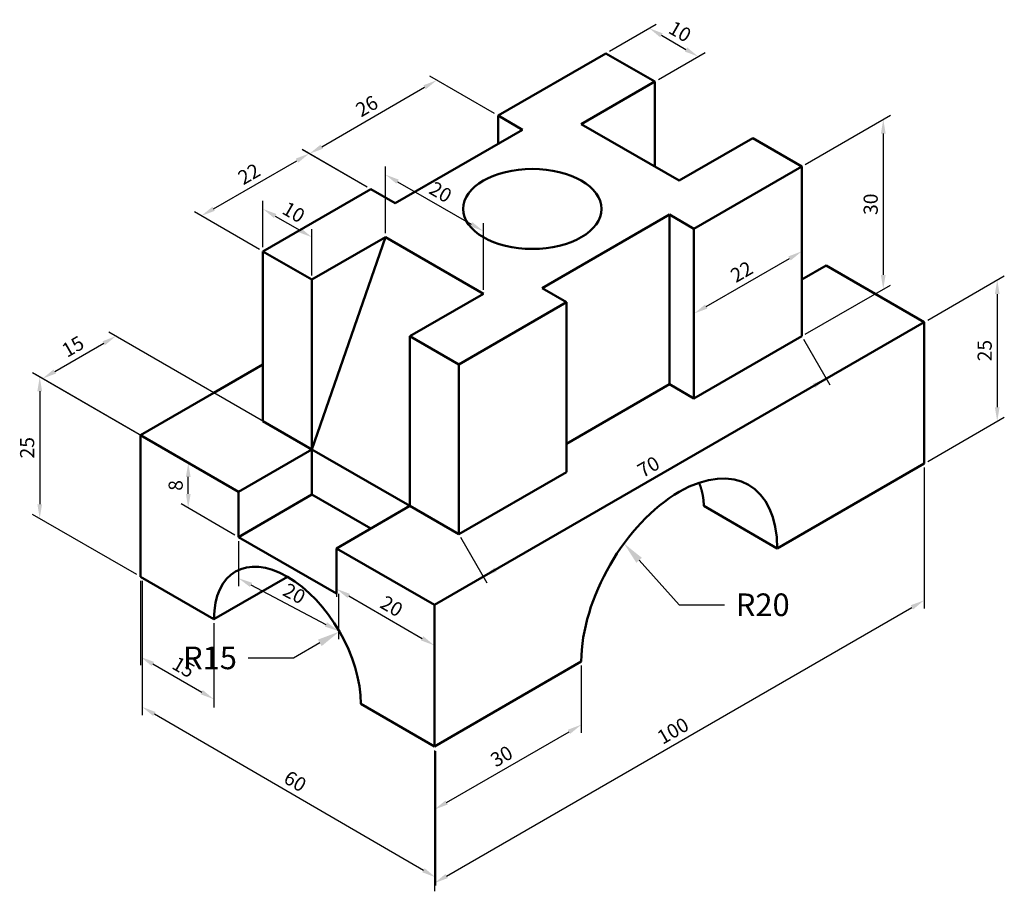
# Model space of a CAD drawing. Units: millimetres. Extents: x 69 to 243, y -4 to 150.
import ezdxf
from ezdxf import colors
from ezdxf.entities.mleader import LeaderData, LeaderLine
from ezdxf.math import Vec2, Vec3

# ---------------------------------------------------------------- set-up
doc = ezdxf.new("R2010")
doc.units = ezdxf.units.MM
for name, color, linetype, lineweight in [('M-DIMS', 3, 'Continuous', 25), ('M-OUTL', 7, 'Continuous', 50), ('M-TEXT', 3, 'Continuous', 25)]:
    doc.layers.add(name, color=color, linetype=linetype, lineweight=lineweight)
doc.styles.get("Standard").update_dxf_attribs({"font": 'arial.ttf'})
doc.dimstyles.new('ISO-25', dxfattribs={"dimtxt": 2.5, "dimasz": 2.5, "dimexe": 1.25, "dimexo": 0.625, "dimtad": 1, "dimtxsty": 'Standard', "dimcen": 2.5, "dimadec": 0, "dimazin": 0, "dimtfac": 1, "dimtmove": 0, "dimatfit": 3, "dimfxl": 1, "dimarcsym": 0})

# ---------------------------------------------------------------- blocks, each defined once
blk = doc.blocks.new('*D1')
at = {"layer": 'Defpoints', "color": 0, "transparency": 16777216}
for p in [(90.55, 76.18), (72.73, 61.47), (90.55, 51.18)]:
    blk.add_point(p, dxfattribs=at)
at = {"layer": 'M-DIMS', "color": 0, "lineweight": -2, "transparency": 16777216}
for p, q in [((89.92, 76.54), (71.48, 87.19)), ((72.73, 83.97), (72.73, 63.97)), ((89.92, 51.54), (71.48, 62.19))]:
    blk.add_line(p, q, dxfattribs=at)
at = {"layer": 'M-DIMS', "color": 0, "transparency": 16777216}
for points in [[(72.32, 83.97), (73.15, 83.97), (72.73, 86.47)], [(72.32, 63.97), (73.15, 63.97), (72.73, 61.47)]]:
    blk.add_solid(points, dxfattribs=at)
at = {"layer": 'M-DIMS', "color": 0, "transparency": 16777216, "insert": (70.83, 73.97), "char_height": 2.5, "attachment_point": 5, "rotation": 90}
blk.add_mtext('25', dxfattribs=at)
blk = doc.blocks.new('*D2')
at = {"layer": 'Defpoints', "color": 0, "transparency": 16777216}
for p in [(90.55, 51.18), (103.54, 43.68), (103.54, 29.51)]:
    blk.add_point(p, dxfattribs=at)
at = {"layer": 'M-DIMS', "color": 0, "lineweight": -2, "transparency": 16777216}
for p, q in [((90.55, 50.46), (90.55, 35.57)), ((103.54, 42.96), (103.54, 28.07)), ((92.71, 35.76), (101.37, 30.76))]:
    blk.add_line(p, q, dxfattribs=at)
at = {"layer": 'M-DIMS', "color": 0, "transparency": 16777216}
for points in [[(92.92, 36.13), (92.51, 35.4), (90.55, 37.01)], [(101.58, 31.13), (101.17, 30.4), (103.54, 29.51)]]:
    blk.add_solid(points, dxfattribs=at)
at = {"layer": 'M-DIMS', "color": 0, "transparency": 16777216, "insert": (98, 34.91), "char_height": 2.5, "attachment_point": 5, "rotation": 330}
blk.add_mtext('15', dxfattribs=at)
blk = doc.blocks.new('*D3')
at = {"layer": 'Defpoints', "color": 0, "transparency": 16777216}
for p in [(90.84, 51.18), (142.73, 21.06), (142.73, -1.96)]:
    blk.add_point(p, dxfattribs=at)
at = {"layer": 'M-DIMS', "color": 0, "lineweight": -2, "transparency": 16777216}
for p, q in [((90.84, 50.46), (90.84, 26.72)), ((93, 26.91), (140.57, -0.7)), ((142.73, 20.33), (142.73, -3.4))]:
    blk.add_line(p, q, dxfattribs=at)
at = {"layer": 'M-DIMS', "color": 0, "transparency": 16777216}
for points in [[(93.21, 27.27), (92.79, 26.55), (90.84, 28.17)], [(140.78, -0.34), (140.36, -1.06), (142.73, -1.96)]]:
    blk.add_solid(points, dxfattribs=at)
at = {"layer": 'M-DIMS', "color": 0, "transparency": 16777216, "insert": (117.74, 14.75), "char_height": 2.5, "attachment_point": 5, "rotation": 329.8606}
blk.add_mtext('60', dxfattribs=at)
blk = doc.blocks.new('*D4')
at = {"layer": 'Defpoints', "color": 0, "transparency": 16777216}
for p in [(168.49, 36.18), (168.49, 25.02), (142.51, 21.18)]:
    blk.add_point(p, dxfattribs=at)
at = {"layer": 'M-DIMS', "color": 0, "lineweight": -2, "transparency": 16777216}
for p, q in [((168.49, 35.46), (168.49, 23.58)), ((144.68, 11.27), (166.33, 23.77)), ((142.51, 20.46), (142.51, 8.58))]:
    blk.add_line(p, q, dxfattribs=at)
at = {"layer": 'M-DIMS', "color": 0, "transparency": 16777216}
for points in [[(166.12, 24.13), (166.53, 23.41), (168.49, 25.02)], [(144.47, 11.63), (144.88, 10.91), (142.51, 10.02)]]:
    blk.add_solid(points, dxfattribs=at)
at = {"layer": 'M-DIMS', "color": 0, "transparency": 16777216, "insert": (154.55, 19.17), "char_height": 2.5, "attachment_point": 5, "rotation": 30}
blk.add_mtext('30', dxfattribs=at)
blk = doc.blocks.new('*D5')
at = {"layer": 'Defpoints', "color": 0, "transparency": 16777216}
for p in [(229.11, 71.18), (229.11, 47.01), (142.51, 21.18)]:
    blk.add_point(p, dxfattribs=at)
at = {"layer": 'M-DIMS', "color": 0, "lineweight": -2, "transparency": 16777216}
for p, q in [((229.11, 70.46), (229.11, 45.57)), ((144.68, -1.74), (226.95, 45.76)), ((142.51, 20.46), (142.51, -4.43))]:
    blk.add_line(p, q, dxfattribs=at)
at = {"layer": 'M-DIMS', "color": 0, "transparency": 16777216}
for points in [[(226.74, 46.13), (227.16, 45.4), (229.11, 47.01)], [(144.47, -1.37), (144.88, -2.1), (142.51, -2.99)]]:
    blk.add_solid(points, dxfattribs=at)
at = {"layer": 'M-DIMS', "color": 0, "transparency": 16777216, "insert": (184.86, 23.66), "char_height": 2.5, "attachment_point": 5, "rotation": 30}
blk.add_mtext('100', dxfattribs=at)
blk = doc.blocks.new('*D6')
at = {"layer": 'Defpoints', "color": 0, "transparency": 16777216}
for p in [(98.99, 71.31), (107.87, 66.18), (107.87, 58.18)]:
    blk.add_point(p, dxfattribs=at)
at = {"layer": 'M-DIMS', "color": 0, "lineweight": -2, "transparency": 16777216}
for p, q in [((107.24, 66.54), (97.74, 72.03)), ((98.99, 65.81), (98.99, 68.81)), ((107.24, 58.54), (97.74, 64.03))]:
    blk.add_line(p, q, dxfattribs=at)
at = {"layer": 'M-DIMS', "color": 0, "transparency": 16777216}
for points in [[(98.58, 68.81), (99.41, 68.81), (98.99, 71.31)], [(98.58, 65.81), (99.41, 65.81), (98.99, 63.31)]]:
    blk.add_solid(points, dxfattribs=at)
at = {"layer": 'M-DIMS', "color": 0, "transparency": 16777216, "insert": (97.09, 67.31), "char_height": 2.5, "attachment_point": 5, "rotation": 90}
blk.add_mtext('8', dxfattribs=at)
blk = doc.blocks.new('*D7')
at = {"layer": 'Defpoints', "color": 0, "transparency": 16777216}
for p in [(86.2, 93.69), (120.86, 73.68), (107.87, 66.18)]:
    blk.add_point(p, dxfattribs=at)
at = {"layer": 'M-DIMS', "color": 0, "lineweight": -2, "transparency": 16777216}
for p, q in [((120.24, 74.04), (84.95, 94.41)), ((75.38, 87.44), (84.04, 92.44)), ((107.24, 66.54), (71.96, 86.91))]:
    blk.add_line(p, q, dxfattribs=at)
at = {"layer": 'M-DIMS', "color": 0, "transparency": 16777216}
for points in [[(83.83, 92.8), (84.25, 92.08), (86.2, 93.69)], [(75.17, 87.8), (75.59, 87.08), (73.21, 86.19)]]:
    blk.add_solid(points, dxfattribs=at)
at = {"layer": 'M-DIMS', "color": 0, "transparency": 16777216, "insert": (78.76, 91.59), "char_height": 2.5, "attachment_point": 5, "rotation": 30}
blk.add_mtext('15', dxfattribs=at)
blk = doc.blocks.new('*D8')
at = {"layer": 'Defpoints', "color": 0, "transparency": 16777216}
for p in [(207.46, 123.68), (221.88, 102.01), (207.46, 93.68)]:
    blk.add_point(p, dxfattribs=at)
at = {"layer": 'M-DIMS', "color": 0, "lineweight": -2, "transparency": 16777216}
for p, q in [((208.09, 124.04), (223.13, 132.73)), ((221.88, 129.51), (221.88, 104.51)), ((208.09, 94.04), (223.13, 102.73))]:
    blk.add_line(p, q, dxfattribs=at)
at = {"layer": 'M-DIMS', "color": 0, "transparency": 16777216}
for points in [[(221.46, 129.51), (222.3, 129.51), (221.88, 132.01)], [(221.46, 104.51), (222.3, 104.51), (221.88, 102.01)]]:
    blk.add_solid(points, dxfattribs=at)
at = {"layer": 'M-DIMS', "color": 0, "transparency": 16777216, "insert": (219.98, 117.01), "char_height": 2.5, "attachment_point": 5, "rotation": 90}
blk.add_mtext('30', dxfattribs=at)
blk = doc.blocks.new('*D9')
at = {"layer": 'Defpoints', "color": 0, "transparency": 16777216}
for p in [(125.19, 56.18), (142.51, 46.18), (142.51, 39.03)]:
    blk.add_point(p, dxfattribs=at)
at = {"layer": 'M-DIMS', "color": 0, "lineweight": -2, "transparency": 16777216}
for p, q in [((125.19, 55.46), (125.19, 47.59)), ((127.36, 47.78), (140.35, 40.28)), ((142.51, 45.46), (142.51, 37.59))]:
    blk.add_line(p, q, dxfattribs=at)
at = {"layer": 'M-DIMS', "color": 0, "transparency": 16777216}
for points in [[(127.56, 48.15), (127.15, 47.42), (125.19, 49.03)], [(140.55, 40.65), (140.14, 39.92), (142.51, 39.03)]]:
    blk.add_solid(points, dxfattribs=at)
at = {"layer": 'M-DIMS', "color": 0, "transparency": 16777216, "insert": (134.8, 45.68), "char_height": 2.5, "attachment_point": 5, "rotation": 330}
blk.add_mtext('20', dxfattribs=at)
blk = doc.blocks.new('*D10')
at = {"layer": 'Defpoints', "color": 0, "transparency": 16777216}
for p in [(107.87, 58.18), (125.56, 48.84), (125.56, 41.57)]:
    blk.add_point(p, dxfattribs=at)
at = {"layer": 'M-DIMS', "color": 0, "lineweight": -2, "transparency": 16777216}
for p, q in [((107.87, 57.47), (107.87, 49.5)), ((110.08, 49.74), (123.34, 42.74)), ((125.56, 48.14), (125.56, 40.16))]:
    blk.add_line(p, q, dxfattribs=at)
at = {"layer": 'M-DIMS', "color": 0, "transparency": 16777216}
for points in [[(110.28, 50.11), (109.89, 49.37), (107.87, 50.91)], [(123.54, 43.11), (123.15, 42.37), (125.56, 41.57)]]:
    blk.add_solid(points, dxfattribs=at)
at = {"layer": 'M-DIMS', "color": 0, "transparency": 16777216, "insert": (117.6, 47.92), "char_height": 2.5, "attachment_point": 5, "rotation": 332.1618}
blk.add_mtext('20', dxfattribs=at)
blk = doc.blocks.new('*D11')
at = {"layer": 'Defpoints', "color": 0, "transparency": 16777216}
for p in [(120.86, 111.18), (112.2, 108.68), (120.86, 103.68)]:
    blk.add_point(p, dxfattribs=at)
at = {"layer": 'M-DIMS', "color": 0, "lineweight": -2, "transparency": 16777216}
for p, q in [((112.2, 109.4), (112.2, 117.63)), ((114.37, 114.93), (118.7, 112.43)), ((120.86, 104.4), (120.86, 112.63))]:
    blk.add_line(p, q, dxfattribs=at)
at = {"layer": 'M-DIMS', "color": 0, "transparency": 16777216}
for points in [[(114.57, 115.29), (114.16, 114.57), (112.2, 116.18)], [(118.9, 112.79), (118.49, 112.07), (120.86, 111.18)]]:
    blk.add_solid(points, dxfattribs=at)
at = {"layer": 'M-DIMS', "color": 0, "transparency": 16777216, "insert": (117.48, 115.33), "char_height": 2.5, "attachment_point": 5, "rotation": 330}
blk.add_mtext('10', dxfattribs=at)
blk = doc.blocks.new('*D12')
at = {"layer": 'Defpoints', "color": 0, "transparency": 16777216}
for p in [(151.17, 112.25), (133.85, 111.18), (151.17, 101.18)]:
    blk.add_point(p, dxfattribs=at)
at = {"layer": 'M-DIMS', "color": 0, "lineweight": -2, "transparency": 16777216}
for p, q in [((133.85, 111.9), (133.85, 123.69)), ((136.02, 121), (149.01, 113.5)), ((151.17, 101.9), (151.17, 113.69))]:
    blk.add_line(p, q, dxfattribs=at)
at = {"layer": 'M-DIMS', "color": 0, "transparency": 16777216}
for points in [[(136.22, 121.36), (135.81, 120.64), (133.85, 122.25)], [(149.21, 113.86), (148.8, 113.14), (151.17, 112.25)]]:
    blk.add_solid(points, dxfattribs=at)
at = {"layer": 'M-DIMS', "color": 0, "transparency": 16777216, "insert": (143.46, 118.89), "char_height": 2.5, "attachment_point": 5, "rotation": 330}
blk.add_mtext('20', dxfattribs=at)
blk = doc.blocks.new('*D13')
at = {"layer": 'Defpoints', "color": 0, "transparency": 16777216}
for p in [(120.37, 125.96), (131.25, 119.68), (112.2, 108.68)]:
    blk.add_point(p, dxfattribs=at)
at = {"layer": 'M-DIMS', "color": 0, "lineweight": -2, "transparency": 16777216}
for p, q in [((130.63, 120.04), (119.12, 126.69)), ((103.48, 116.21), (118.21, 124.71)), ((111.58, 109.04), (100.07, 115.69))]:
    blk.add_line(p, q, dxfattribs=at)
at = {"layer": 'M-DIMS', "color": 0, "transparency": 16777216}
for points in [[(118, 125.08), (118.41, 124.35), (120.37, 125.96)], [(103.27, 116.58), (103.69, 115.85), (101.32, 114.96)]]:
    blk.add_solid(points, dxfattribs=at)
at = {"layer": 'M-DIMS', "color": 0, "transparency": 16777216, "insert": (109.9, 122.09), "char_height": 2.5, "attachment_point": 5, "rotation": 30}
blk.add_mtext('22', dxfattribs=at)
blk = doc.blocks.new('*D14')
at = {"layer": 'Defpoints', "color": 0, "transparency": 16777216}
for p in [(142.94, 138.93), (153.77, 132.68), (131.25, 119.68)]:
    blk.add_point(p, dxfattribs=at)
at = {"layer": 'M-DIMS', "color": 0, "lineweight": -2, "transparency": 16777216}
for p, q in [((153.14, 133.04), (141.69, 139.65)), ((122.59, 127.18), (140.78, 137.68)), ((130.63, 120.04), (119.17, 126.65))]:
    blk.add_line(p, q, dxfattribs=at)
at = {"layer": 'M-DIMS', "color": 0, "transparency": 16777216}
for points in [[(140.57, 138.04), (140.98, 137.32), (142.94, 138.93)], [(122.38, 127.54), (122.8, 126.82), (120.42, 125.93)]]:
    blk.add_solid(points, dxfattribs=at)
at = {"layer": 'M-DIMS', "color": 0, "transparency": 16777216, "insert": (130.73, 134.08), "char_height": 2.5, "attachment_point": 5, "rotation": 30}
blk.add_mtext('26', dxfattribs=at)
blk = doc.blocks.new('*D15')
at = {"layer": 'Defpoints', "color": 0, "transparency": 16777216}
for p in [(207.46, 93.68), (211.79, 86.18), (146.84, 58.68)]:
    blk.add_point(p, dxfattribs=at)
at = {"layer": 'M-DIMS', "color": 0, "lineweight": -2, "transparency": 16777216}
for p, q in [((207.78, 93.14), (212.42, 85.1)), ((153.34, 52.43), (209.63, 84.93)), ((147.15, 58.14), (151.8, 50.1))]:
    blk.add_line(p, q, dxfattribs=at)
at = {"layer": 'M-DIMS', "color": 0, "transparency": 16777216}
for points in [[(209.42, 85.29), (209.84, 84.57), (211.79, 86.18)], [(153.13, 52.79), (153.54, 52.07), (151.17, 51.18)]]:
    blk.add_solid(points, dxfattribs=at)
at = {"layer": 'M-DIMS', "color": 0, "transparency": 16777216, "insert": (180.53, 70.33), "char_height": 2.5, "attachment_point": 5, "rotation": 30}
blk.add_mtext('70', dxfattribs=at)
blk = doc.blocks.new('*D16')
at = {"layer": 'Defpoints', "color": 0, "transparency": 16777216}
for p in [(207.46, 108.68), (207.46, 93.68), (188.41, 82.68)]:
    blk.add_point(p, dxfattribs=at)
at = {"layer": 'M-DIMS', "color": 0, "lineweight": -2, "transparency": 16777216}
for p, q in [((207.46, 94.4), (207.46, 110.13)), ((190.58, 98.93), (205.3, 107.43)), ((188.41, 83.4), (188.41, 99.13))]:
    blk.add_line(p, q, dxfattribs=at)
at = {"layer": 'M-DIMS', "color": 0, "transparency": 16777216}
for points in [[(205.09, 107.79), (205.51, 107.07), (207.46, 108.68)], [(190.37, 99.29), (190.78, 98.57), (188.41, 97.68)]]:
    blk.add_solid(points, dxfattribs=at)
at = {"layer": 'M-DIMS', "color": 0, "transparency": 16777216, "insert": (197, 104.81), "char_height": 2.5, "attachment_point": 5, "rotation": 30}
blk.add_mtext('22', dxfattribs=at)
blk = doc.blocks.new('*D17')
at = {"layer": 'Defpoints', "color": 0, "transparency": 16777216}
for p in [(229.11, 96.18), (242.03, 78.64), (229.11, 71.18)]:
    blk.add_point(p, dxfattribs=at)
at = {"layer": 'M-DIMS', "color": 0, "lineweight": -2, "transparency": 16777216}
for p, q in [((229.74, 96.54), (243.28, 104.36)), ((242.03, 101.14), (242.03, 81.14)), ((229.74, 71.54), (243.28, 79.36))]:
    blk.add_line(p, q, dxfattribs=at)
at = {"layer": 'M-DIMS', "color": 0, "transparency": 16777216}
for points in [[(241.61, 101.14), (242.45, 101.14), (242.03, 103.64)], [(241.61, 81.14), (242.45, 81.14), (242.03, 78.64)]]:
    blk.add_solid(points, dxfattribs=at)
at = {"layer": 'M-DIMS', "color": 0, "transparency": 16777216, "insert": (240.13, 91.14), "char_height": 2.5, "attachment_point": 5, "rotation": 90}
blk.add_mtext('25', dxfattribs=at)
blk = doc.blocks.new('*D18')
at = {"layer": 'Defpoints', "color": 0, "transparency": 16777216}
for p in [(172.82, 143.68), (189.16, 143.12), (181.48, 138.68)]:
    blk.add_point(p, dxfattribs=at)
at = {"layer": 'M-DIMS', "color": 0, "lineweight": -2, "transparency": 16777216}
for p, q in [((173.45, 144.04), (181.75, 148.84)), ((182.67, 146.87), (187, 144.37)), ((182.11, 139.04), (190.41, 143.84))]:
    blk.add_line(p, q, dxfattribs=at)
at = {"layer": 'M-DIMS', "color": 0, "transparency": 16777216}
for points in [[(182.87, 147.23), (182.46, 146.5), (180.5, 148.12)], [(187.2, 144.73), (186.79, 144), (189.16, 143.12)]]:
    blk.add_solid(points, dxfattribs=at)
at = {"layer": 'M-DIMS', "color": 0, "transparency": 16777216, "insert": (185.78, 147.26), "char_height": 2.5, "attachment_point": 5, "rotation": 330}
blk.add_mtext('10', dxfattribs=at)

msp = doc.modelspace()

# ---------------------------------------------------------------- linework, layer by layer
at = {"layer": 'M-OUTL'}
for p, q in [((153.769, 132.682), (172.822, 143.682)), ((172.822, 143.682), (181.482, 138.682)), ((181.482, 138.682), (168.492, 131.182)), ((181.482, 138.682), (181.482, 123.682)), ((158.099, 130.182), (153.769, 132.682)), ((153.769, 132.682), (153.769, 127.682)), ((168.492, 131.182), (185.812, 121.182)), ((135.583, 117.182), (158.099, 130.182)), ((185.812, 121.182), (198.803, 128.682)), ((198.803, 128.682), (207.463, 123.682)), ((188.41, 112.682), (207.463, 123.682)), ((207.463, 123.682), (207.463, 93.682)), ((112.2, 108.682), (131.253, 119.682)), ((131.253, 119.682), (135.583, 117.182)), ((161.564, 102.182), (184.08, 115.182)), ((184.08, 115.182), (188.41, 112.682)), ((184.08, 115.182), (184.08, 85.182)), ((188.41, 82.682), (188.41, 112.682)), ((120.86, 103.682), (133.851, 111.182)), ((133.851, 111.182), (120.86, 73.682)), ((133.851, 111.182), (151.171, 101.182)), ((112.2, 78.682), (112.2, 108.682)), ((112.2, 108.682), (120.86, 103.682)), ((211.793, 106.182), (207.463, 103.682)), ((229.114, 96.182), (211.793, 106.182)), ((120.86, 103.682), (120.86, 73.682)), ((151.171, 101.182), (138.181, 93.682)), ((165.894, 99.682), (161.564, 102.182)), ((165.894, 99.682), (146.841, 88.682)), ((165.894, 69.682), (165.894, 99.682)), ((142.511, 46.182), (229.114, 96.182)), ((229.114, 96.182), (229.114, 71.182)), ((138.181, 93.682), (146.841, 88.682)), ((138.181, 93.682), (138.181, 63.682)), ((207.463, 93.682), (188.41, 82.682)), ((103.54, 83.682), (112.2, 88.682)), ((146.841, 88.682), (146.841, 58.682)), ((90.549, 76.182), (103.54, 83.682)), ((184.08, 85.182), (165.894, 74.682)), ((184.08, 85.182), (188.41, 82.682)), ((112.2, 78.682), (120.86, 73.682)), ((90.549, 51.182), (90.549, 76.182)), ((90.549, 76.182), (107.87, 66.182)), ((107.87, 66.182), (120.86, 73.682)), ((120.86, 73.682), (138.181, 63.682)), ((120.86, 73.682), (120.86, 65.682)), ((146.841, 58.682), (165.894, 69.682)), ((203.133, 56.182), (229.114, 71.182)), ((107.87, 66.182), (107.87, 58.182)), ((120.86, 65.682), (107.87, 58.182)), ((120.86, 65.682), (131.253, 59.682)), ((138.181, 63.682), (125.19, 56.182)), ((138.181, 63.682), (146.841, 58.682)), ((203.132, 56.182), (190.142, 63.682)), ((107.87, 58.182), (125.19, 48.182)), ((125.19, 48.182), (125.19, 56.182)), ((125.19, 56.182), (142.511, 46.182)), ((90.549, 51.182), (103.54, 43.682)), ((103.539, 43.682), (116.53, 51.182)), ((142.511, 46.182), (142.511, 21.182)), ((142.511, 21.182), (168.492, 36.182)), ((129.521, 28.682), (142.511, 21.182))]:
    msp.add_line(p, q, dxfattribs=at)
msp.add_lwpolyline([(189.307, 67.788), (189.323, 67.748), (189.339, 67.707), (189.356, 67.666), (189.372, 67.625), (189.387, 67.584), (189.403, 67.543), (189.419, 67.502), (189.434, 67.461), (189.45, 67.42), (189.465, 67.378), (189.48, 67.337), (189.495, 67.296), (189.509, 67.254), (189.524, 67.213), (189.538, 67.171), (189.552, 67.129), (189.567, 67.088), (189.581, 67.046), (189.594, 67.004), (189.608, 66.962), (189.621, 66.921), (189.635, 66.879), (189.648, 66.837), (189.661, 66.795), (189.674, 66.753), (189.686, 66.711), (189.699, 66.668), (189.711, 66.626), (189.724, 66.584), (189.736, 66.542), (189.748, 66.499), (189.759, 66.457), (189.771, 66.414), (189.782, 66.372), (189.793, 66.329), (189.805, 66.287), (189.815, 66.244), (189.826, 66.202), (189.837, 66.159), (189.847, 66.116), (189.857, 66.073), (189.867, 66.031), (189.877, 65.988), (189.887, 65.945), (189.896, 65.902), (189.906, 65.859), (189.915, 65.816), (189.924, 65.773), (189.933, 65.73), (189.942, 65.687), (189.95, 65.644), (189.958, 65.601), (189.966, 65.557), (189.974, 65.514), (189.982, 65.471), (189.99, 65.428), (189.997, 65.385), (190.004, 65.341), (190.011, 65.298), (190.018, 65.255), (190.025, 65.211), (190.032, 65.168), (190.038, 65.124), (190.044, 65.081), (190.05, 65.037), (190.056, 64.994), (190.061, 64.95), (190.067, 64.907), (190.072, 64.863), (190.077, 64.82), (190.082, 64.776), (190.087, 64.732), (190.091, 64.689), (190.095, 64.645), (190.1, 64.601), (190.103, 64.558), (190.107, 64.514), (190.111, 64.47), (190.114, 64.427), (190.117, 64.383), (190.12, 64.339), (190.123, 64.295), (190.126, 64.252), (190.128, 64.208), (190.13, 64.164), (190.132, 64.12), (190.134, 64.076), (190.136, 64.033), (190.137, 63.989), (190.138, 63.945), (190.14, 63.901), (190.14, 63.857), (190.141, 63.814), (190.142, 63.77), (190.142, 63.726), (190.142, 63.682)], dxfattribs=at)
msp.add_ellipse((159.831, 116.182), major_axis=(-12.247, 0), ratio=0.5773503, dxfattribs=at)
for centre, major_axis, start_param, end_param in [((185.812, 46.182), (-12.247, -21.213), 2.3561945, 5.4977871), ((116.53, 36.182), (9.186, -15.91), 0.7853982, 3.9269908)]:
    msp.add_ellipse(centre, major_axis=major_axis, ratio=0.5773503, start_param=start_param, end_param=end_param, dxfattribs=at)

# ---------------------------------------------------------------- dimensions: what is measured, and where the dimension line sits
at = {"layer": 'M-DIMS'}
for p1, p2, distance, picture, middle in [((172.822, 143.682), (181.482, 138.682), 7.679, '*D18', (185.782, 147.262)), ((131.253, 119.682), (153.769, 132.682), 10.828, '*D14', (130.733, 134.08)), ((207.463, 123.682), (207.463, 93.682), 14.419, '*D8', (219.979, 117.006)), ((112.2, 108.682), (131.253, 119.682), 10.882, '*D13', (109.904, 122.093)), ((133.851, 111.182), (151.171, 101.182), 9.582, '*D12', (143.462, 118.893)), ((112.2, 108.682), (120.86, 103.682), 6.495, '*D11', (117.481, 115.328)), ((188.41, 82.682), (207.463, 93.682), 12.99, '*D16', (196.997, 104.81)), ((229.114, 96.182), (229.114, 71.182), 12.917, '*D17', (240.129, 91.139)), ((107.87, 66.182), (120.86, 73.682), 34.656, '*D7', (78.758, 91.587)), ((146.841, 58.682), (207.463, 93.682), -8.66, '*D15', (180.531, 70.328)), ((90.549, 76.182), (90.549, 51.182), -17.817, '*D1', (70.831, 73.968)), ((107.87, 58.182), (107.87, 66.182), 8.876, '*D6', (97.093, 67.306)), ((142.511, 21.182), (229.114, 71.182), -20.93, '*D5', (184.862, 23.661)), ((107.87, 58.182), (125.555, 48.842), -6.431, '*D10', (117.601, 47.921)), ((125.19, 56.182), (142.511, 46.182), -6.189, '*D9', (134.801, 45.682)), ((90.549, 51.182), (103.54, 43.682), -12.269, '*D2', (97.995, 34.912)), ((90.84, 51.182), (142.729, 21.055), -19.901, '*D3', (117.739, 14.751)), ((142.511, 21.182), (168.492, 36.182), -9.665, '*D4', (154.55, 19.169))]:
    dim = msp.add_aligned_dim(p1=p1, p2=p2, distance=distance, dimstyle='ISO-25', override={"dimclrd": 0, "dimclre": 0, "dimclrt": 0}, dxfattribs=at)
    dim.commit()
    dim.dimension.update_dxf_attribs({"geometry": picture, "text_midpoint": middle})

# ---------------------------------------------------------------- leaders
at = {"layer": 'M-TEXT'}
ml = msp.add_multileader_mtext('Standard', dxfattribs=at)
ml.set_content('R20', color=256)
ml.set_leader_properties()
ml.build(insert=Vec2(0, 0))
ctx = ml.context
ctx.base_point, ctx.plane_origin = Vec3(193.812, 46.182), Vec3(176.037, 57.048)
notes = []
notes.append((ctx, [(0, (1, 1, 0), (185.812, 46.182), (1, 0), 8, [(0, [(176.037, 57.048)], 0, [])])]))
ctx.mtext.insert, ctx.mtext.flow_direction = Vec3(195.812, 48.216), 5
ml = msp.add_multileader_mtext('Standard', dxfattribs=at)
ml.set_content('R15', color=256)
ml.set_leader_properties()
ml.build(insert=Vec2(0, 0))
ctx = ml.context
ctx.base_point, ctx.plane_origin = Vec3(96.008, 36.797), Vec3(125.716, 41.485)
ctx.text_align_type = 2
notes.append((ctx, [(0, (1, 1, 0), (117.596, 36.797), (-1, 0), 8, [(0, [(125.716, 41.485)], 0, [])])]))
ctx.mtext.insert, ctx.mtext.alignment, ctx.mtext.flow_direction = Vec3(107.596, 38.831), 3, 5
for ctx, leaders in notes:
    for number, flags, end, landing, length, lines in leaders:
        leader = LeaderData()
        leader.index, (leader.has_last_leader_line, leader.has_dogleg_vector, leader.attachment_direction) = number, flags
        leader.last_leader_point, leader.dogleg_vector, leader.dogleg_length = Vec3(end), Vec3(landing), length
        for number, points, colour, breaks in lines:
            line = LeaderLine()
            line.index, line.vertices, line.color, line.breaks = number, Vec3.list(points), colors.encode_raw_color(colour), breaks
            leader.lines.append(line)
        ctx.leaders.append(leader)

doc.saveas('drawing.dxf')
